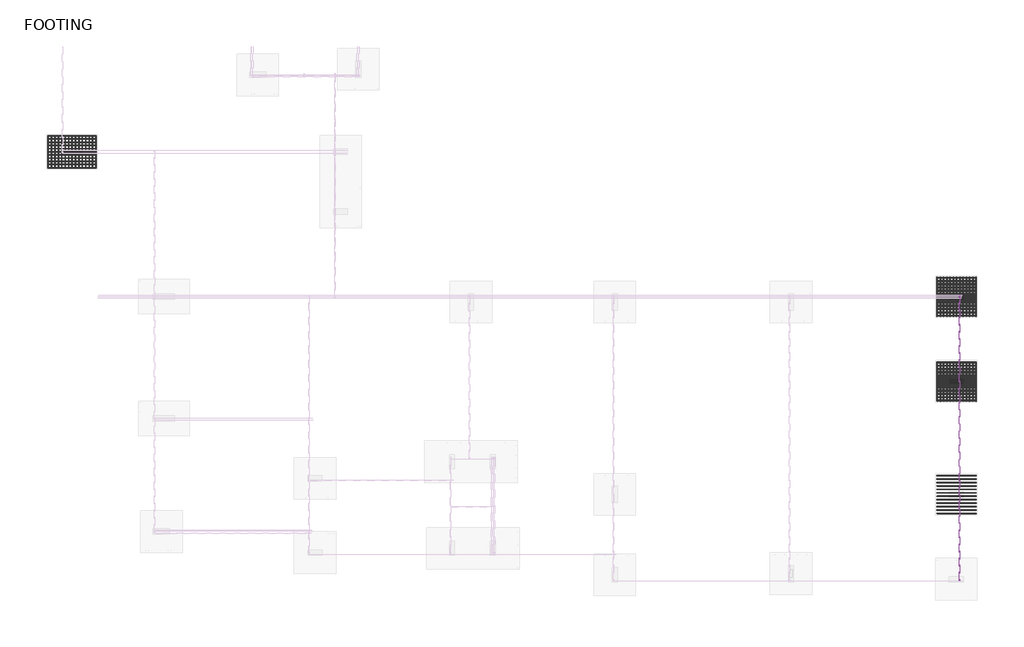
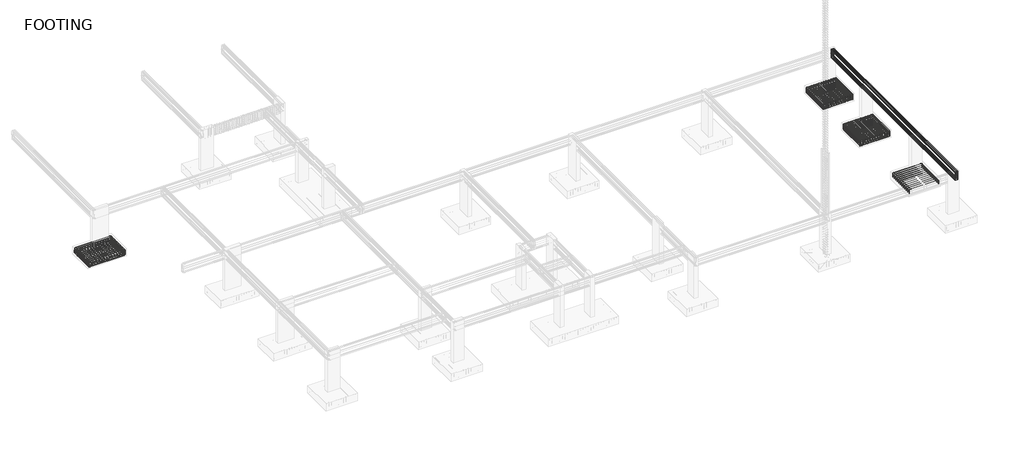
# One storey, part 9 of 12: 15 reinforcing bars.
"""IFC4 building model written with IfcOpenShell, lengths in millimetres."""

from ifc_helpers import new_model, si_unit, point, frame, origin, place, context, project, spatial, polyline, circle_curve, trimmed, segment, composite_curve, source, transform, mapped, element, save
from ifc_brep_helpers import swept_disk

model = new_model("IFC4")

# Units and contexts
model_context = context("Model", 3, world=origin())
ifc_project = project(units=[si_unit("LENGTHUNIT", "METRE", prefix="MILLI")], contexts=[model_context])

# Site, building, storey
site = spatial("IfcSite", under=ifc_project)
building = spatial("IfcBuilding", under=site)
storey = spatial("IfcBuildingStorey", under=building, Name="FOOTING", Elevation=-5638.8)

# Reinforcing bars
placement = place(None, origin())
reinforcing_bar_shape = source(origin(), model_context, "Body", "SolidModel", [
    swept_disk(composite_curve([segment(polyline([(18367.9998335, -9883.6399866, -5950.85), (18367.9998335, -9883.6399866, -5764.25)]), True, "CONTINUOUS"), segment(trimmed(circle_curve(frame((18423.4498335, -9883.6399866, -5764.25), z_axis=(0.0, 1.0, 0.0), x_axis=(-55.45000000000073, 0.0, 0.0)), 55.45), [point((18367.9998335, -9883.6399866, -5764.25))], [point((18423.4498335, -9883.6399866, -5708.8))], True, "CARTESIAN"), True, "CONTINUOUS"), segment(polyline([(18423.4498335, -9883.6399866, -5708.8), (19996.6498335, -9883.6399866, -5708.8)]), True, "CONTINUOUS"), segment(trimmed(circle_curve(frame((19996.6498335, -9883.6399866, -5764.25), z_axis=(0.0, 1.0, 0.0), x_axis=(0.0, 0.0, 55.44999999999982)), 55.45), [point((19996.6498335, -9883.6399866, -5708.8))], [point((20052.0998335, -9883.6399866, -5764.25))], True, "CARTESIAN"), True, "CONTINUOUS"), segment(polyline([(20052.0998335, -9883.6399866, -5764.25), (20052.0998335, -9883.6399866, -5950.85)]), True, "CONTINUOUS")], self_intersect=False), 7.95),
])
element("IfcReinforcingBar", 1, at=placement, inside=storey, context=model_context, shape_type="MappedRepresentation", body=[
    mapped(reinforcing_bar_shape, transform((0.0, 0.0, 0.0), x_axis=(1.0, 0.0, 0.0), y_axis=(0.0, 1.0, 0.0), z_axis=(0.0, 0.0, 1.0))),
    mapped(reinforcing_bar_shape, transform((0.0, -148.1882348, 0.0), x_axis=(1.0, 0.0, 0.0), y_axis=(0.0, 1.0, 0.0), z_axis=(0.0, 0.0, 1.0))),
    mapped(reinforcing_bar_shape, transform((0.0, -296.3764695, 0.0), x_axis=(1.0, 0.0, 0.0), y_axis=(0.0, 1.0, 0.0), z_axis=(0.0, 0.0, 1.0))),
    mapped(reinforcing_bar_shape, transform((0.0, -444.5647043, 0.0), x_axis=(1.0, 0.0, 0.0), y_axis=(0.0, 1.0, 0.0), z_axis=(0.0, 0.0, 1.0))),
    mapped(reinforcing_bar_shape, transform((0.0, -592.7529391, 0.0), x_axis=(1.0, 0.0, 0.0), y_axis=(0.0, 1.0, 0.0), z_axis=(0.0, 0.0, 1.0))),
    mapped(reinforcing_bar_shape, transform((0.0, -740.9411738, 0.0), x_axis=(1.0, 0.0, 0.0), y_axis=(0.0, 1.0, 0.0), z_axis=(0.0, 0.0, 1.0))),
    mapped(reinforcing_bar_shape, transform((0.0, -889.1294086, 0.0), x_axis=(1.0, 0.0, 0.0), y_axis=(0.0, 1.0, 0.0), z_axis=(0.0, 0.0, 1.0))),
    mapped(reinforcing_bar_shape, transform((0.0, -1037.3176434, 0.0), x_axis=(1.0, 0.0, 0.0), y_axis=(0.0, 1.0, 0.0), z_axis=(0.0, 0.0, 1.0))),
    mapped(reinforcing_bar_shape, transform((0.0, -1185.5058782, 0.0), x_axis=(1.0, 0.0, 0.0), y_axis=(0.0, 1.0, 0.0), z_axis=(0.0, 0.0, 1.0))),
    mapped(reinforcing_bar_shape, transform((0.0, -1333.6941129, 0.0), x_axis=(1.0, 0.0, 0.0), y_axis=(0.0, 1.0, 0.0), z_axis=(0.0, 0.0, 1.0))),
    mapped(reinforcing_bar_shape, transform((0.0, -1481.8823477, 0.0), x_axis=(1.0, 0.0, 0.0), y_axis=(0.0, 1.0, 0.0), z_axis=(0.0, 0.0, 1.0))),
    mapped(reinforcing_bar_shape, transform((0.0, -1630.0705825, 0.0), x_axis=(1.0, 0.0, 0.0), y_axis=(0.0, 1.0, 0.0), z_axis=(0.0, 0.0, 1.0))),
])
reinforcing_bar_2_shape = source(origin(), model_context, "Body", "SolidModel", [
    swept_disk(composite_curve([segment(polyline([(20052.0998335, -6666.5541655, -5788.8), (20052.0998335, -6666.5541655, -5975.4)]), True, "CONTINUOUS"), segment(trimmed(circle_curve(frame((20052.0998335, -6611.1041655, -5975.4), z_axis=(1.0, 0.0, 0.0), x_axis=(0.0, -55.44999999999982, 0.0)), 55.45), [point((20052.0998335, -6666.5541655, -5975.4))], [point((20052.0998335, -6611.1041655, -6030.85))], True, "CARTESIAN"), True, "CONTINUOUS"), segment(polyline([(20052.0998335, -6611.1041655, -6030.85), (20052.0998335, -5037.9041655, -6030.85)]), True, "CONTINUOUS"), segment(trimmed(circle_curve(frame((20052.0998335, -5037.9041655, -5975.4), z_axis=(1.0, 0.0, 0.0), x_axis=(0.0, 0.0, -55.45000000000073)), 55.45), [point((20052.0998335, -5037.9041655, -6030.85))], [point((20052.0998335, -4982.4541655, -5975.4))], True, "CARTESIAN"), True, "CONTINUOUS"), segment(polyline([(20052.0998335, -4982.4541655, -5975.4), (20052.0998335, -4982.4541655, -5788.8)]), True, "CONTINUOUS")], self_intersect=False), 7.95),
])
element("IfcReinforcingBar", 2, at=placement, inside=storey, context=model_context, shape_type="MappedRepresentation", body=[
    mapped(reinforcing_bar_2_shape, transform((0.0, 0.0, 0.0), x_axis=(1.0, 0.0, 0.0), y_axis=(0.0, 1.0, 0.0), z_axis=(0.0, 0.0, 1.0))),
    mapped(reinforcing_bar_2_shape, transform((-140.3416667, 0.0, 0.0), x_axis=(1.0, 0.0, 0.0), y_axis=(0.0, 1.0, 0.0), z_axis=(0.0, 0.0, 1.0))),
    mapped(reinforcing_bar_2_shape, transform((-280.6833333, 0.0, 0.0), x_axis=(1.0, 0.0, 0.0), y_axis=(0.0, 1.0, 0.0), z_axis=(0.0, 0.0, 1.0))),
    mapped(reinforcing_bar_2_shape, transform((-421.025, 0.0, 0.0), x_axis=(1.0, 0.0, 0.0), y_axis=(0.0, 1.0, 0.0), z_axis=(0.0, 0.0, 1.0))),
    mapped(reinforcing_bar_2_shape, transform((-561.3666667, 0.0, 0.0), x_axis=(1.0, 0.0, 0.0), y_axis=(0.0, 1.0, 0.0), z_axis=(0.0, 0.0, 1.0))),
    mapped(reinforcing_bar_2_shape, transform((-701.7083333, 0.0, 0.0), x_axis=(1.0, 0.0, 0.0), y_axis=(0.0, 1.0, 0.0), z_axis=(0.0, 0.0, 1.0))),
    mapped(reinforcing_bar_2_shape, transform((-842.05, 0.0, 0.0), x_axis=(1.0, 0.0, 0.0), y_axis=(0.0, 1.0, 0.0), z_axis=(0.0, 0.0, 1.0))),
    mapped(reinforcing_bar_2_shape, transform((-982.3916667, 0.0, 0.0), x_axis=(1.0, 0.0, 0.0), y_axis=(0.0, 1.0, 0.0), z_axis=(0.0, 0.0, 1.0))),
    mapped(reinforcing_bar_2_shape, transform((-1122.7333333, 0.0, 0.0), x_axis=(1.0, 0.0, 0.0), y_axis=(0.0, 1.0, 0.0), z_axis=(0.0, 0.0, 1.0))),
    mapped(reinforcing_bar_2_shape, transform((-1263.075, 0.0, 0.0), x_axis=(1.0, 0.0, 0.0), y_axis=(0.0, 1.0, 0.0), z_axis=(0.0, 0.0, 1.0))),
    mapped(reinforcing_bar_2_shape, transform((-1403.4166667, 0.0, 0.0), x_axis=(1.0, 0.0, 0.0), y_axis=(0.0, 1.0, 0.0), z_axis=(0.0, 0.0, 1.0))),
    mapped(reinforcing_bar_2_shape, transform((-1543.7583333, 0.0, 0.0), x_axis=(1.0, 0.0, 0.0), y_axis=(0.0, 1.0, 0.0), z_axis=(0.0, 0.0, 1.0))),
    mapped(reinforcing_bar_2_shape, transform((-1684.1, 0.0, 0.0), x_axis=(1.0, 0.0, 0.0), y_axis=(0.0, 1.0, 0.0), z_axis=(0.0, 0.0, 1.0))),
])
reinforcing_bar_3_shape = source(origin(), model_context, "Body", "SolidModel", [
    swept_disk(composite_curve([segment(polyline([(20042.9597994, -4980.8541655, -5888.8), (20042.9597994, -4980.8541655, -5741.5)]), True, "CONTINUOUS"), segment(trimmed(circle_curve(frame((20042.9597994, -5027.2041655, -5741.5), z_axis=(1.0, 0.0, 0.0), x_axis=(0.0, 46.350000000000364, 0.0)), 46.35), [point((20042.9597994, -4980.8541655, -5741.5))], [point((20042.9597994, -5027.2041655, -5695.15))], True, "CARTESIAN"), True, "CONTINUOUS"), segment(polyline([(20042.9597994, -5027.2041655, -5695.15), (20042.9597994, -6621.8041655, -5695.15)]), True, "CONTINUOUS"), segment(trimmed(circle_curve(frame((20042.9597994, -6621.8041655, -5741.5), z_axis=(1.0, 0.0, 0.0), x_axis=(0.0, 0.0, 46.350000000000364)), 46.35), [point((20042.9597994, -6621.8041655, -5695.15))], [point((20042.9597994, -6668.1541655, -5741.5))], True, "CARTESIAN"), True, "CONTINUOUS"), segment(polyline([(20042.9597994, -6668.1541655, -5741.5), (20042.9597994, -6668.1541655, -5888.8)]), True, "CONTINUOUS")], self_intersect=False), 6.35),
])
element("IfcReinforcingBar", 3, at=placement, inside=storey, context=model_context, shape_type="MappedRepresentation", body=[
    mapped(reinforcing_bar_3_shape, transform((0.0, 0.0, 0.0), x_axis=(1.0, 0.0, 0.0), y_axis=(0.0, 1.0, 0.0), z_axis=(0.0, 0.0, 1.0))),
    mapped(reinforcing_bar_3_shape, transform((-138.4829293, 0.0, 0.0), x_axis=(1.0, 0.0, 0.0), y_axis=(0.0, 1.0, 0.0), z_axis=(0.0, 0.0, 1.0))),
    mapped(reinforcing_bar_3_shape, transform((-276.9658586, 0.0, 0.0), x_axis=(1.0, 0.0, 0.0), y_axis=(0.0, 1.0, 0.0), z_axis=(0.0, 0.0, 1.0))),
    mapped(reinforcing_bar_3_shape, transform((-415.4487879, 0.0, 0.0), x_axis=(1.0, 0.0, 0.0), y_axis=(0.0, 1.0, 0.0), z_axis=(0.0, 0.0, 1.0))),
    mapped(reinforcing_bar_3_shape, transform((-553.9317172, 0.0, 0.0), x_axis=(1.0, 0.0, 0.0), y_axis=(0.0, 1.0, 0.0), z_axis=(0.0, 0.0, 1.0))),
    mapped(reinforcing_bar_3_shape, transform((-692.4146465, 0.0, 0.0), x_axis=(1.0, 0.0, 0.0), y_axis=(0.0, 1.0, 0.0), z_axis=(0.0, 0.0, 1.0))),
    mapped(reinforcing_bar_3_shape, transform((-830.8975758, 0.0, 0.0), x_axis=(1.0, 0.0, 0.0), y_axis=(0.0, 1.0, 0.0), z_axis=(0.0, 0.0, 1.0))),
    mapped(reinforcing_bar_3_shape, transform((-969.3805051, 0.0, 0.0), x_axis=(1.0, 0.0, 0.0), y_axis=(0.0, 1.0, 0.0), z_axis=(0.0, 0.0, 1.0))),
    mapped(reinforcing_bar_3_shape, transform((-1107.8634344, 0.0, 0.0), x_axis=(1.0, 0.0, 0.0), y_axis=(0.0, 1.0, 0.0), z_axis=(0.0, 0.0, 1.0))),
    mapped(reinforcing_bar_3_shape, transform((-1246.3463637, 0.0, 0.0), x_axis=(1.0, 0.0, 0.0), y_axis=(0.0, 1.0, 0.0), z_axis=(0.0, 0.0, 1.0))),
    mapped(reinforcing_bar_3_shape, transform((-1384.8292929, 0.0, 0.0), x_axis=(1.0, 0.0, 0.0), y_axis=(0.0, 1.0, 0.0), z_axis=(0.0, 0.0, 1.0))),
    mapped(reinforcing_bar_3_shape, transform((-1523.3122222, 0.0, 0.0), x_axis=(1.0, 0.0, 0.0), y_axis=(0.0, 1.0, 0.0), z_axis=(0.0, 0.0, 1.0))),
    mapped(reinforcing_bar_3_shape, transform((-1661.7951515, 0.0, 0.0), x_axis=(1.0, 0.0, 0.0), y_axis=(0.0, 1.0, 0.0), z_axis=(0.0, 0.0, 1.0))),
])
reinforcing_bar_4_shape = source(origin(), model_context, "Body", "SolidModel", [
    swept_disk(composite_curve([segment(polyline([(18367.9998335, -6649.5041655, -5773.0), (18367.9998335, -6649.5041655, -5959.6)]), True, "CONTINUOUS"), segment(trimmed(circle_curve(frame((18423.4498335, -6649.5041655, -5959.6), z_axis=(0.0, -1.0, 0.0), x_axis=(-55.45000000000073, 0.0, 0.0)), 55.45), [point((18367.9998335, -6649.5041655, -5959.6))], [point((18423.4498335, -6649.5041655, -6015.05))], True, "CARTESIAN"), True, "CONTINUOUS"), segment(polyline([(18423.4498335, -6649.5041655, -6015.05), (19996.6498335, -6649.5041655, -6015.05)]), True, "CONTINUOUS"), segment(trimmed(circle_curve(frame((19996.6498335, -6649.5041655, -5959.6), z_axis=(0.0, -1.0, 0.0), x_axis=(0.0, 0.0, -55.44999999999982)), 55.45), [point((19996.6498335, -6649.5041655, -6015.05))], [point((20052.0998335, -6649.5041655, -5959.6))], True, "CARTESIAN"), True, "CONTINUOUS"), segment(polyline([(20052.0998335, -6649.5041655, -5959.6), (20052.0998335, -6649.5041655, -5773.0)]), True, "CONTINUOUS")], self_intersect=False), 7.95),
])
element("IfcReinforcingBar", 4, at=placement, inside=storey, context=model_context, shape_type="MappedRepresentation", body=[
    mapped(reinforcing_bar_4_shape, transform((0.0, 0.0, 0.0), x_axis=(1.0, 0.0, 0.0), y_axis=(0.0, 1.0, 0.0), z_axis=(0.0, 0.0, 1.0))),
    mapped(reinforcing_bar_4_shape, transform((0.0, 137.7402087, 0.0), x_axis=(1.0, 0.0, 0.0), y_axis=(0.0, 1.0, 0.0), z_axis=(0.0, 0.0, 1.0))),
    mapped(reinforcing_bar_4_shape, transform((0.0, 275.4804175, 0.0), x_axis=(1.0, 0.0, 0.0), y_axis=(0.0, 1.0, 0.0), z_axis=(0.0, 0.0, 1.0))),
    mapped(reinforcing_bar_4_shape, transform((0.0, 413.2206262, 0.0), x_axis=(1.0, 0.0, 0.0), y_axis=(0.0, 1.0, 0.0), z_axis=(0.0, 0.0, 1.0))),
    mapped(reinforcing_bar_4_shape, transform((0.0, 550.960835, 0.0), x_axis=(1.0, 0.0, 0.0), y_axis=(0.0, 1.0, 0.0), z_axis=(0.0, 0.0, 1.0))),
    mapped(reinforcing_bar_4_shape, transform((0.0, 688.7010437, 0.0), x_axis=(1.0, 0.0, 0.0), y_axis=(0.0, 1.0, 0.0), z_axis=(0.0, 0.0, 1.0))),
    mapped(reinforcing_bar_4_shape, transform((0.0, 826.4412525, 0.0), x_axis=(1.0, 0.0, 0.0), y_axis=(0.0, 1.0, 0.0), z_axis=(0.0, 0.0, 1.0))),
    mapped(reinforcing_bar_4_shape, transform((0.0, 964.1814612, 0.0), x_axis=(1.0, 0.0, 0.0), y_axis=(0.0, 1.0, 0.0), z_axis=(0.0, 0.0, 1.0))),
    mapped(reinforcing_bar_4_shape, transform((0.0, 1101.92167, 0.0), x_axis=(1.0, 0.0, 0.0), y_axis=(0.0, 1.0, 0.0), z_axis=(0.0, 0.0, 1.0))),
    mapped(reinforcing_bar_4_shape, transform((0.0, 1239.6618787, 0.0), x_axis=(1.0, 0.0, 0.0), y_axis=(0.0, 1.0, 0.0), z_axis=(0.0, 0.0, 1.0))),
    mapped(reinforcing_bar_4_shape, transform((0.0, 1377.4020875, 0.0), x_axis=(1.0, 0.0, 0.0), y_axis=(0.0, 1.0, 0.0), z_axis=(0.0, 0.0, 1.0))),
    mapped(reinforcing_bar_4_shape, transform((0.0, 1515.1422962, 0.0), x_axis=(1.0, 0.0, 0.0), y_axis=(0.0, 1.0, 0.0), z_axis=(0.0, 0.0, 1.0))),
    mapped(reinforcing_bar_4_shape, transform((0.0, 1652.882505, 0.0), x_axis=(1.0, 0.0, 0.0), y_axis=(0.0, 1.0, 0.0), z_axis=(0.0, 0.0, 1.0))),
])
reinforcing_bar_5_shape = source(origin(), model_context, "Body", "SolidModel", [
    swept_disk(composite_curve([segment(polyline([(18367.9998335, -5006.8399866, -5950.85), (18367.9998335, -5006.8399866, -5764.25)]), True, "CONTINUOUS"), segment(trimmed(circle_curve(frame((18423.4498335, -5006.8399866, -5764.25), z_axis=(0.0, 1.0, 0.0), x_axis=(-55.45000000000073, 0.0, 0.0)), 55.45), [point((18367.9998335, -5006.8399866, -5764.25))], [point((18423.4498335, -5006.8399866, -5708.8))], True, "CARTESIAN"), True, "CONTINUOUS"), segment(polyline([(18423.4498335, -5006.8399866, -5708.8), (19996.6498335, -5006.8399866, -5708.8)]), True, "CONTINUOUS"), segment(trimmed(circle_curve(frame((19996.6498335, -5006.8399866, -5764.25), z_axis=(0.0, 1.0, 0.0), x_axis=(0.0, 0.0, 55.44999999999982)), 55.45), [point((19996.6498335, -5006.8399866, -5708.8))], [point((20052.0998335, -5006.8399866, -5764.25))], True, "CARTESIAN"), True, "CONTINUOUS"), segment(polyline([(20052.0998335, -5006.8399866, -5764.25), (20052.0998335, -5006.8399866, -5950.85)]), True, "CONTINUOUS")], self_intersect=False), 7.95),
])
element("IfcReinforcingBar", 5, at=placement, inside=storey, context=model_context, shape_type="MappedRepresentation", body=[
    mapped(reinforcing_bar_5_shape, transform((0.0, 0.0, 0.0), x_axis=(1.0, 0.0, 0.0), y_axis=(0.0, 1.0, 0.0), z_axis=(0.0, 0.0, 1.0))),
    mapped(reinforcing_bar_5_shape, transform((0.0, -148.1882348, 0.0), x_axis=(1.0, 0.0, 0.0), y_axis=(0.0, 1.0, 0.0), z_axis=(0.0, 0.0, 1.0))),
    mapped(reinforcing_bar_5_shape, transform((0.0, -296.3764695, 0.0), x_axis=(1.0, 0.0, 0.0), y_axis=(0.0, 1.0, 0.0), z_axis=(0.0, 0.0, 1.0))),
    mapped(reinforcing_bar_5_shape, transform((0.0, -444.5647043, 0.0), x_axis=(1.0, 0.0, 0.0), y_axis=(0.0, 1.0, 0.0), z_axis=(0.0, 0.0, 1.0))),
    mapped(reinforcing_bar_5_shape, transform((0.0, -592.7529391, 0.0), x_axis=(1.0, 0.0, 0.0), y_axis=(0.0, 1.0, 0.0), z_axis=(0.0, 0.0, 1.0))),
    mapped(reinforcing_bar_5_shape, transform((0.0, -740.9411738, 0.0), x_axis=(1.0, 0.0, 0.0), y_axis=(0.0, 1.0, 0.0), z_axis=(0.0, 0.0, 1.0))),
    mapped(reinforcing_bar_5_shape, transform((0.0, -889.1294086, 0.0), x_axis=(1.0, 0.0, 0.0), y_axis=(0.0, 1.0, 0.0), z_axis=(0.0, 0.0, 1.0))),
    mapped(reinforcing_bar_5_shape, transform((0.0, -1037.3176434, 0.0), x_axis=(1.0, 0.0, 0.0), y_axis=(0.0, 1.0, 0.0), z_axis=(0.0, 0.0, 1.0))),
    mapped(reinforcing_bar_5_shape, transform((0.0, -1185.5058782, 0.0), x_axis=(1.0, 0.0, 0.0), y_axis=(0.0, 1.0, 0.0), z_axis=(0.0, 0.0, 1.0))),
    mapped(reinforcing_bar_5_shape, transform((0.0, -1333.6941129, 0.0), x_axis=(1.0, 0.0, 0.0), y_axis=(0.0, 1.0, 0.0), z_axis=(0.0, 0.0, 1.0))),
    mapped(reinforcing_bar_5_shape, transform((0.0, -1481.8823477, 0.0), x_axis=(1.0, 0.0, 0.0), y_axis=(0.0, 1.0, 0.0), z_axis=(0.0, 0.0, 1.0))),
    mapped(reinforcing_bar_5_shape, transform((0.0, -1630.0705825, 0.0), x_axis=(1.0, 0.0, 0.0), y_axis=(0.0, 1.0, 0.0), z_axis=(0.0, 0.0, 1.0))),
])
reinforcing_bar_6_shape = source(origin(), model_context, "Body", "SolidModel", [
    swept_disk(composite_curve([segment(polyline([(20052.0998335, -3008.9541655, -5788.8), (20052.0998335, -3008.9541655, -5975.4)]), True, "CONTINUOUS"), segment(trimmed(circle_curve(frame((20052.0998335, -2953.5041655, -5975.4), z_axis=(1.0, 0.0, 0.0), x_axis=(0.0, -55.44999999999982, 0.0)), 55.45), [point((20052.0998335, -3008.9541655, -5975.4))], [point((20052.0998335, -2953.5041655, -6030.85))], True, "CARTESIAN"), True, "CONTINUOUS"), segment(polyline([(20052.0998335, -2953.5041655, -6030.85), (20052.0998335, -1380.3041655, -6030.85)]), True, "CONTINUOUS"), segment(trimmed(circle_curve(frame((20052.0998335, -1380.3041655, -5975.4), z_axis=(1.0, 0.0, 0.0), x_axis=(0.0, 0.0, -55.45000000000073)), 55.45), [point((20052.0998335, -1380.3041655, -6030.85))], [point((20052.0998335, -1324.8541655, -5975.4))], True, "CARTESIAN"), True, "CONTINUOUS"), segment(polyline([(20052.0998335, -1324.8541655, -5975.4), (20052.0998335, -1324.8541655, -5788.8)]), True, "CONTINUOUS")], self_intersect=False), 7.95),
])
element("IfcReinforcingBar", 6, at=placement, inside=storey, context=model_context, shape_type="MappedRepresentation", body=[
    mapped(reinforcing_bar_6_shape, transform((0.0, 0.0, 0.0), x_axis=(1.0, 0.0, 0.0), y_axis=(0.0, 1.0, 0.0), z_axis=(0.0, 0.0, 1.0))),
    mapped(reinforcing_bar_6_shape, transform((-140.3416667, 0.0, 0.0), x_axis=(1.0, 0.0, 0.0), y_axis=(0.0, 1.0, 0.0), z_axis=(0.0, 0.0, 1.0))),
    mapped(reinforcing_bar_6_shape, transform((-280.6833333, 0.0, 0.0), x_axis=(1.0, 0.0, 0.0), y_axis=(0.0, 1.0, 0.0), z_axis=(0.0, 0.0, 1.0))),
    mapped(reinforcing_bar_6_shape, transform((-421.025, 0.0, 0.0), x_axis=(1.0, 0.0, 0.0), y_axis=(0.0, 1.0, 0.0), z_axis=(0.0, 0.0, 1.0))),
    mapped(reinforcing_bar_6_shape, transform((-561.3666667, 0.0, 0.0), x_axis=(1.0, 0.0, 0.0), y_axis=(0.0, 1.0, 0.0), z_axis=(0.0, 0.0, 1.0))),
    mapped(reinforcing_bar_6_shape, transform((-701.7083333, 0.0, 0.0), x_axis=(1.0, 0.0, 0.0), y_axis=(0.0, 1.0, 0.0), z_axis=(0.0, 0.0, 1.0))),
    mapped(reinforcing_bar_6_shape, transform((-842.05, 0.0, 0.0), x_axis=(1.0, 0.0, 0.0), y_axis=(0.0, 1.0, 0.0), z_axis=(0.0, 0.0, 1.0))),
    mapped(reinforcing_bar_6_shape, transform((-982.3916667, 0.0, 0.0), x_axis=(1.0, 0.0, 0.0), y_axis=(0.0, 1.0, 0.0), z_axis=(0.0, 0.0, 1.0))),
    mapped(reinforcing_bar_6_shape, transform((-1122.7333333, 0.0, 0.0), x_axis=(1.0, 0.0, 0.0), y_axis=(0.0, 1.0, 0.0), z_axis=(0.0, 0.0, 1.0))),
    mapped(reinforcing_bar_6_shape, transform((-1263.075, 0.0, 0.0), x_axis=(1.0, 0.0, 0.0), y_axis=(0.0, 1.0, 0.0), z_axis=(0.0, 0.0, 1.0))),
    mapped(reinforcing_bar_6_shape, transform((-1403.4166667, 0.0, 0.0), x_axis=(1.0, 0.0, 0.0), y_axis=(0.0, 1.0, 0.0), z_axis=(0.0, 0.0, 1.0))),
    mapped(reinforcing_bar_6_shape, transform((-1543.7583333, 0.0, 0.0), x_axis=(1.0, 0.0, 0.0), y_axis=(0.0, 1.0, 0.0), z_axis=(0.0, 0.0, 1.0))),
    mapped(reinforcing_bar_6_shape, transform((-1684.1, 0.0, 0.0), x_axis=(1.0, 0.0, 0.0), y_axis=(0.0, 1.0, 0.0), z_axis=(0.0, 0.0, 1.0))),
])
reinforcing_bar_7_shape = source(origin(), model_context, "Body", "SolidModel", [
    swept_disk(composite_curve([segment(polyline([(20042.9597994, -1323.2541655, -5888.8), (20042.9597994, -1323.2541655, -5741.5)]), True, "CONTINUOUS"), segment(trimmed(circle_curve(frame((20042.9597994, -1369.6041655, -5741.5), z_axis=(1.0, 0.0, 0.0), x_axis=(0.0, 46.34999999999991, 0.0)), 46.35), [point((20042.9597994, -1323.2541655, -5741.5))], [point((20042.9597994, -1369.6041655, -5695.15))], True, "CARTESIAN"), True, "CONTINUOUS"), segment(polyline([(20042.9597994, -1369.6041655, -5695.15), (20042.9597994, -2964.2041655, -5695.15)]), True, "CONTINUOUS"), segment(trimmed(circle_curve(frame((20042.9597994, -2964.2041655, -5741.5), z_axis=(1.0, 0.0, 0.0), x_axis=(0.0, 0.0, 46.350000000000364)), 46.35), [point((20042.9597994, -2964.2041655, -5695.15))], [point((20042.9597994, -3010.5541655, -5741.5))], True, "CARTESIAN"), True, "CONTINUOUS"), segment(polyline([(20042.9597994, -3010.5541655, -5741.5), (20042.9597994, -3010.5541655, -5888.8)]), True, "CONTINUOUS")], self_intersect=False), 6.35),
])
element("IfcReinforcingBar", 7, at=placement, inside=storey, context=model_context, shape_type="MappedRepresentation", body=[
    mapped(reinforcing_bar_7_shape, transform((0.0, 0.0, 0.0), x_axis=(1.0, 0.0, 0.0), y_axis=(0.0, 1.0, 0.0), z_axis=(0.0, 0.0, 1.0))),
    mapped(reinforcing_bar_7_shape, transform((-138.4829293, 0.0, 0.0), x_axis=(1.0, 0.0, 0.0), y_axis=(0.0, 1.0, 0.0), z_axis=(0.0, 0.0, 1.0))),
    mapped(reinforcing_bar_7_shape, transform((-276.9658586, 0.0, 0.0), x_axis=(1.0, 0.0, 0.0), y_axis=(0.0, 1.0, 0.0), z_axis=(0.0, 0.0, 1.0))),
    mapped(reinforcing_bar_7_shape, transform((-415.4487879, 0.0, 0.0), x_axis=(1.0, 0.0, 0.0), y_axis=(0.0, 1.0, 0.0), z_axis=(0.0, 0.0, 1.0))),
    mapped(reinforcing_bar_7_shape, transform((-553.9317172, 0.0, 0.0), x_axis=(1.0, 0.0, 0.0), y_axis=(0.0, 1.0, 0.0), z_axis=(0.0, 0.0, 1.0))),
    mapped(reinforcing_bar_7_shape, transform((-692.4146465, 0.0, 0.0), x_axis=(1.0, 0.0, 0.0), y_axis=(0.0, 1.0, 0.0), z_axis=(0.0, 0.0, 1.0))),
    mapped(reinforcing_bar_7_shape, transform((-830.8975758, 0.0, 0.0), x_axis=(1.0, 0.0, 0.0), y_axis=(0.0, 1.0, 0.0), z_axis=(0.0, 0.0, 1.0))),
    mapped(reinforcing_bar_7_shape, transform((-969.3805051, 0.0, 0.0), x_axis=(1.0, 0.0, 0.0), y_axis=(0.0, 1.0, 0.0), z_axis=(0.0, 0.0, 1.0))),
    mapped(reinforcing_bar_7_shape, transform((-1107.8634344, 0.0, 0.0), x_axis=(1.0, 0.0, 0.0), y_axis=(0.0, 1.0, 0.0), z_axis=(0.0, 0.0, 1.0))),
    mapped(reinforcing_bar_7_shape, transform((-1246.3463637, 0.0, 0.0), x_axis=(1.0, 0.0, 0.0), y_axis=(0.0, 1.0, 0.0), z_axis=(0.0, 0.0, 1.0))),
    mapped(reinforcing_bar_7_shape, transform((-1384.8292929, 0.0, 0.0), x_axis=(1.0, 0.0, 0.0), y_axis=(0.0, 1.0, 0.0), z_axis=(0.0, 0.0, 1.0))),
    mapped(reinforcing_bar_7_shape, transform((-1523.3122222, 0.0, 0.0), x_axis=(1.0, 0.0, 0.0), y_axis=(0.0, 1.0, 0.0), z_axis=(0.0, 0.0, 1.0))),
    mapped(reinforcing_bar_7_shape, transform((-1661.7951515, 0.0, 0.0), x_axis=(1.0, 0.0, 0.0), y_axis=(0.0, 1.0, 0.0), z_axis=(0.0, 0.0, 1.0))),
])
reinforcing_bar_8_shape = source(origin(), model_context, "Body", "SolidModel", [
    swept_disk(composite_curve([segment(polyline([(18367.9998335, -2991.9041655, -5773.0), (18367.9998335, -2991.9041655, -5959.6)]), True, "CONTINUOUS"), segment(trimmed(circle_curve(frame((18423.4498335, -2991.9041655, -5959.6), z_axis=(0.0, -1.0, 0.0), x_axis=(-55.45000000000073, 0.0, 0.0)), 55.45), [point((18367.9998335, -2991.9041655, -5959.6))], [point((18423.4498335, -2991.9041655, -6015.05))], True, "CARTESIAN"), True, "CONTINUOUS"), segment(polyline([(18423.4498335, -2991.9041655, -6015.05), (19996.6498335, -2991.9041655, -6015.05)]), True, "CONTINUOUS"), segment(trimmed(circle_curve(frame((19996.6498335, -2991.9041655, -5959.6), z_axis=(0.0, -1.0, 0.0), x_axis=(0.0, 0.0, -55.44999999999982)), 55.45), [point((19996.6498335, -2991.9041655, -6015.05))], [point((20052.0998335, -2991.9041655, -5959.6))], True, "CARTESIAN"), True, "CONTINUOUS"), segment(polyline([(20052.0998335, -2991.9041655, -5959.6), (20052.0998335, -2991.9041655, -5773.0)]), True, "CONTINUOUS")], self_intersect=False), 7.95),
])
element("IfcReinforcingBar", 8, at=placement, inside=storey, context=model_context, shape_type="MappedRepresentation", body=[
    mapped(reinforcing_bar_8_shape, transform((0.0, 0.0, 0.0), x_axis=(1.0, 0.0, 0.0), y_axis=(0.0, 1.0, 0.0), z_axis=(0.0, 0.0, 1.0))),
    mapped(reinforcing_bar_8_shape, transform((0.0, 137.7402087, 0.0), x_axis=(1.0, 0.0, 0.0), y_axis=(0.0, 1.0, 0.0), z_axis=(0.0, 0.0, 1.0))),
    mapped(reinforcing_bar_8_shape, transform((0.0, 275.4804175, 0.0), x_axis=(1.0, 0.0, 0.0), y_axis=(0.0, 1.0, 0.0), z_axis=(0.0, 0.0, 1.0))),
    mapped(reinforcing_bar_8_shape, transform((0.0, 413.2206262, 0.0), x_axis=(1.0, 0.0, 0.0), y_axis=(0.0, 1.0, 0.0), z_axis=(0.0, 0.0, 1.0))),
    mapped(reinforcing_bar_8_shape, transform((0.0, 550.960835, 0.0), x_axis=(1.0, 0.0, 0.0), y_axis=(0.0, 1.0, 0.0), z_axis=(0.0, 0.0, 1.0))),
    mapped(reinforcing_bar_8_shape, transform((0.0, 688.7010437, 0.0), x_axis=(1.0, 0.0, 0.0), y_axis=(0.0, 1.0, 0.0), z_axis=(0.0, 0.0, 1.0))),
    mapped(reinforcing_bar_8_shape, transform((0.0, 826.4412525, 0.0), x_axis=(1.0, 0.0, 0.0), y_axis=(0.0, 1.0, 0.0), z_axis=(0.0, 0.0, 1.0))),
    mapped(reinforcing_bar_8_shape, transform((0.0, 964.1814612, 0.0), x_axis=(1.0, 0.0, 0.0), y_axis=(0.0, 1.0, 0.0), z_axis=(0.0, 0.0, 1.0))),
    mapped(reinforcing_bar_8_shape, transform((0.0, 1101.92167, 0.0), x_axis=(1.0, 0.0, 0.0), y_axis=(0.0, 1.0, 0.0), z_axis=(0.0, 0.0, 1.0))),
    mapped(reinforcing_bar_8_shape, transform((0.0, 1239.6618787, 0.0), x_axis=(1.0, 0.0, 0.0), y_axis=(0.0, 1.0, 0.0), z_axis=(0.0, 0.0, 1.0))),
    mapped(reinforcing_bar_8_shape, transform((0.0, 1377.4020875, 0.0), x_axis=(1.0, 0.0, 0.0), y_axis=(0.0, 1.0, 0.0), z_axis=(0.0, 0.0, 1.0))),
    mapped(reinforcing_bar_8_shape, transform((0.0, 1515.1422962, 0.0), x_axis=(1.0, 0.0, 0.0), y_axis=(0.0, 1.0, 0.0), z_axis=(0.0, 0.0, 1.0))),
    mapped(reinforcing_bar_8_shape, transform((0.0, 1652.882505, 0.0), x_axis=(1.0, 0.0, 0.0), y_axis=(0.0, 1.0, 0.0), z_axis=(0.0, 0.0, 1.0))),
])
reinforcing_bar_9_shape = source(origin(), model_context, "Body", "SolidModel", [
    swept_disk(composite_curve([segment(polyline([(18367.9998335, -1349.2399866, -5950.85), (18367.9998335, -1349.2399866, -5764.25)]), True, "CONTINUOUS"), segment(trimmed(circle_curve(frame((18423.4498335, -1349.2399866, -5764.25), z_axis=(0.0, 1.0, 0.0), x_axis=(-55.45000000000073, 0.0, 0.0)), 55.45), [point((18367.9998335, -1349.2399866, -5764.25))], [point((18423.4498335, -1349.2399866, -5708.8))], True, "CARTESIAN"), True, "CONTINUOUS"), segment(polyline([(18423.4498335, -1349.2399866, -5708.8), (19996.6498335, -1349.2399866, -5708.8)]), True, "CONTINUOUS"), segment(trimmed(circle_curve(frame((19996.6498335, -1349.2399866, -5764.25), z_axis=(0.0, 1.0, 0.0), x_axis=(0.0, 0.0, 55.44999999999982)), 55.45), [point((19996.6498335, -1349.2399866, -5708.8))], [point((20052.0998335, -1349.2399866, -5764.25))], True, "CARTESIAN"), True, "CONTINUOUS"), segment(polyline([(20052.0998335, -1349.2399866, -5764.25), (20052.0998335, -1349.2399866, -5950.85)]), True, "CONTINUOUS")], self_intersect=False), 7.95),
])
element("IfcReinforcingBar", 9, at=placement, inside=storey, context=model_context, shape_type="MappedRepresentation", body=[
    mapped(reinforcing_bar_9_shape, transform((0.0, 0.0, 0.0), x_axis=(1.0, 0.0, 0.0), y_axis=(0.0, 1.0, 0.0), z_axis=(0.0, 0.0, 1.0))),
    mapped(reinforcing_bar_9_shape, transform((0.0, -148.1882348, 0.0), x_axis=(1.0, 0.0, 0.0), y_axis=(0.0, 1.0, 0.0), z_axis=(0.0, 0.0, 1.0))),
    mapped(reinforcing_bar_9_shape, transform((0.0, -296.3764695, 0.0), x_axis=(1.0, 0.0, 0.0), y_axis=(0.0, 1.0, 0.0), z_axis=(0.0, 0.0, 1.0))),
    mapped(reinforcing_bar_9_shape, transform((0.0, -444.5647043, 0.0), x_axis=(1.0, 0.0, 0.0), y_axis=(0.0, 1.0, 0.0), z_axis=(0.0, 0.0, 1.0))),
    mapped(reinforcing_bar_9_shape, transform((0.0, -592.7529391, 0.0), x_axis=(1.0, 0.0, 0.0), y_axis=(0.0, 1.0, 0.0), z_axis=(0.0, 0.0, 1.0))),
    mapped(reinforcing_bar_9_shape, transform((0.0, -740.9411738, 0.0), x_axis=(1.0, 0.0, 0.0), y_axis=(0.0, 1.0, 0.0), z_axis=(0.0, 0.0, 1.0))),
    mapped(reinforcing_bar_9_shape, transform((0.0, -889.1294086, 0.0), x_axis=(1.0, 0.0, 0.0), y_axis=(0.0, 1.0, 0.0), z_axis=(0.0, 0.0, 1.0))),
    mapped(reinforcing_bar_9_shape, transform((0.0, -1037.3176434, 0.0), x_axis=(1.0, 0.0, 0.0), y_axis=(0.0, 1.0, 0.0), z_axis=(0.0, 0.0, 1.0))),
    mapped(reinforcing_bar_9_shape, transform((0.0, -1185.5058782, 0.0), x_axis=(1.0, 0.0, 0.0), y_axis=(0.0, 1.0, 0.0), z_axis=(0.0, 0.0, 1.0))),
    mapped(reinforcing_bar_9_shape, transform((0.0, -1333.6941129, 0.0), x_axis=(1.0, 0.0, 0.0), y_axis=(0.0, 1.0, 0.0), z_axis=(0.0, 0.0, 1.0))),
    mapped(reinforcing_bar_9_shape, transform((0.0, -1481.8823477, 0.0), x_axis=(1.0, 0.0, 0.0), y_axis=(0.0, 1.0, 0.0), z_axis=(0.0, 0.0, 1.0))),
    mapped(reinforcing_bar_9_shape, transform((0.0, -1630.0705825, 0.0), x_axis=(1.0, 0.0, 0.0), y_axis=(0.0, 1.0, 0.0), z_axis=(0.0, 0.0, 1.0))),
])
reinforcing_bar_10_shape = source(origin(), model_context, "Body", "SolidModel", [
    swept_disk(composite_curve([segment(polyline([(-19946.3001665, 3387.8458345, -5837.6659404), (-19946.3001665, 3387.8458345, -5984.9659404)]), True, "CONTINUOUS"), segment(trimmed(circle_curve(frame((-19899.9501665, 3387.8458345, -5984.9659404), z_axis=(0.0, -1.0, 0.0), x_axis=(-46.35000000000218, 0.0, 0.0)), 46.35), [point((-19946.3001665, 3387.8458345, -5984.9659404))], [point((-19899.9501665, 3387.8458345, -6031.3159404))], True, "CARTESIAN"), True, "CONTINUOUS"), segment(polyline([(-19899.9501665, 3387.8458345, -6031.3159404), (-17905.3501665, 3387.8458345, -6031.3159404)]), True, "CONTINUOUS"), segment(trimmed(circle_curve(frame((-17905.3501665, 3387.8458345, -5984.9659404), z_axis=(0.0, -1.0, 0.0), x_axis=(0.0, 0.0, -46.349999999999454)), 46.35), [point((-17905.3501665, 3387.8458345, -6031.3159404))], [point((-17859.0001665, 3387.8458345, -5984.9659404))], True, "CARTESIAN"), True, "CONTINUOUS"), segment(polyline([(-17859.0001665, 3387.8458345, -5984.9659404), (-17859.0001665, 3387.8458345, -5837.6659404)]), True, "CONTINUOUS")], self_intersect=False), 6.35),
])
element("IfcReinforcingBar", 10, at=placement, inside=storey, context=model_context, shape_type="MappedRepresentation", body=[
    mapped(reinforcing_bar_10_shape, transform((0.0, 0.0, 0.0), x_axis=(1.0, 0.0, 0.0), y_axis=(0.0, 1.0, 0.0), z_axis=(0.0, 0.0, 1.0))),
    mapped(reinforcing_bar_10_shape, transform((0.0, 138.73, 0.0), x_axis=(1.0, 0.0, 0.0), y_axis=(0.0, 1.0, 0.0), z_axis=(0.0, 0.0, 1.0))),
    mapped(reinforcing_bar_10_shape, transform((0.0, 277.46, 0.0), x_axis=(1.0, 0.0, 0.0), y_axis=(0.0, 1.0, 0.0), z_axis=(0.0, 0.0, 1.0))),
    mapped(reinforcing_bar_10_shape, transform((0.0, 416.19, 0.0), x_axis=(1.0, 0.0, 0.0), y_axis=(0.0, 1.0, 0.0), z_axis=(0.0, 0.0, 1.0))),
    mapped(reinforcing_bar_10_shape, transform((0.0, 554.92, 0.0), x_axis=(1.0, 0.0, 0.0), y_axis=(0.0, 1.0, 0.0), z_axis=(0.0, 0.0, 1.0))),
    mapped(reinforcing_bar_10_shape, transform((0.0, 693.65, 0.0), x_axis=(1.0, 0.0, 0.0), y_axis=(0.0, 1.0, 0.0), z_axis=(0.0, 0.0, 1.0))),
    mapped(reinforcing_bar_10_shape, transform((0.0, 832.38, 0.0), x_axis=(1.0, 0.0, 0.0), y_axis=(0.0, 1.0, 0.0), z_axis=(0.0, 0.0, 1.0))),
    mapped(reinforcing_bar_10_shape, transform((0.0, 971.11, 0.0), x_axis=(1.0, 0.0, 0.0), y_axis=(0.0, 1.0, 0.0), z_axis=(0.0, 0.0, 1.0))),
    mapped(reinforcing_bar_10_shape, transform((0.0, 1109.84, 0.0), x_axis=(1.0, 0.0, 0.0), y_axis=(0.0, 1.0, 0.0), z_axis=(0.0, 0.0, 1.0))),
    mapped(reinforcing_bar_10_shape, transform((0.0, 1248.57, 0.0), x_axis=(1.0, 0.0, 0.0), y_axis=(0.0, 1.0, 0.0), z_axis=(0.0, 0.0, 1.0))),
    mapped(reinforcing_bar_10_shape, transform((0.0, 1387.3, 0.0), x_axis=(1.0, 0.0, 0.0), y_axis=(0.0, 1.0, 0.0), z_axis=(0.0, 0.0, 1.0))),
])
reinforcing_bar_11_shape = source(origin(), model_context, "Body", "SolidModel", [
    swept_disk(composite_curve([segment(polyline([(-17859.0001665, 3400.6454807, -5888.8), (-17859.0001665, 3400.6454807, -5741.5)]), True, "CONTINUOUS"), segment(trimmed(circle_curve(frame((-17905.3501665, 3400.6454807, -5741.5), z_axis=(0.0, -1.0, 0.0), x_axis=(46.349999999998545, 0.0, 0.0)), 46.35), [point((-17859.0001665, 3400.6454807, -5741.5))], [point((-17905.3501665, 3400.6454807, -5695.15))], True, "CARTESIAN"), True, "CONTINUOUS"), segment(polyline([(-17905.3501665, 3400.6454807, -5695.15), (-19899.9501665, 3400.6454807, -5695.15)]), True, "CONTINUOUS"), segment(trimmed(circle_curve(frame((-19899.9501665, 3400.6454807, -5741.5), z_axis=(0.0, -1.0, 0.0), x_axis=(0.0, 0.0, 46.350000000000364)), 46.35), [point((-19899.9501665, 3400.6454807, -5695.15))], [point((-19946.3001665, 3400.6454807, -5741.5))], True, "CARTESIAN"), True, "CONTINUOUS"), segment(polyline([(-19946.3001665, 3400.6454807, -5741.5), (-19946.3001665, 3400.6454807, -5888.8)]), True, "CONTINUOUS")], self_intersect=False), 6.35),
])
element("IfcReinforcingBar", 11, at=placement, inside=storey, context=model_context, shape_type="MappedRepresentation", body=[
    mapped(reinforcing_bar_11_shape, transform((0.0, 0.0, 0.0), x_axis=(1.0, 0.0, 0.0), y_axis=(0.0, 1.0, 0.0), z_axis=(0.0, 0.0, 1.0))),
    mapped(reinforcing_bar_11_shape, transform((0.0, 136.1586067, 0.0), x_axis=(1.0, 0.0, 0.0), y_axis=(0.0, 1.0, 0.0), z_axis=(0.0, 0.0, 1.0))),
    mapped(reinforcing_bar_11_shape, transform((0.0, 272.3172133, 0.0), x_axis=(1.0, 0.0, 0.0), y_axis=(0.0, 1.0, 0.0), z_axis=(0.0, 0.0, 1.0))),
    mapped(reinforcing_bar_11_shape, transform((0.0, 408.47582, 0.0), x_axis=(1.0, 0.0, 0.0), y_axis=(0.0, 1.0, 0.0), z_axis=(0.0, 0.0, 1.0))),
    mapped(reinforcing_bar_11_shape, transform((0.0, 544.6344267, 0.0), x_axis=(1.0, 0.0, 0.0), y_axis=(0.0, 1.0, 0.0), z_axis=(0.0, 0.0, 1.0))),
    mapped(reinforcing_bar_11_shape, transform((0.0, 680.7930333, 0.0), x_axis=(1.0, 0.0, 0.0), y_axis=(0.0, 1.0, 0.0), z_axis=(0.0, 0.0, 1.0))),
    mapped(reinforcing_bar_11_shape, transform((0.0, 816.95164, 0.0), x_axis=(1.0, 0.0, 0.0), y_axis=(0.0, 1.0, 0.0), z_axis=(0.0, 0.0, 1.0))),
    mapped(reinforcing_bar_11_shape, transform((0.0, 953.1102467, 0.0), x_axis=(1.0, 0.0, 0.0), y_axis=(0.0, 1.0, 0.0), z_axis=(0.0, 0.0, 1.0))),
    mapped(reinforcing_bar_11_shape, transform((0.0, 1089.2688533, 0.0), x_axis=(1.0, 0.0, 0.0), y_axis=(0.0, 1.0, 0.0), z_axis=(0.0, 0.0, 1.0))),
    mapped(reinforcing_bar_11_shape, transform((0.0, 1225.42746, 0.0), x_axis=(1.0, 0.0, 0.0), y_axis=(0.0, 1.0, 0.0), z_axis=(0.0, 0.0, 1.0))),
    mapped(reinforcing_bar_11_shape, transform((0.0, 1361.5860667, 0.0), x_axis=(1.0, 0.0, 0.0), y_axis=(0.0, 1.0, 0.0), z_axis=(0.0, 0.0, 1.0))),
])
reinforcing_bar_12_shape = source(origin(), model_context, "Body", "SolidModel", [
    swept_disk(composite_curve([segment(polyline([(-19934.3866414, 4775.1458345, -5821.490176), (-19934.3866414, 4775.1458345, -5968.790176)]), True, "CONTINUOUS"), segment(trimmed(circle_curve(frame((-19934.3866414, 4728.7958345, -5968.790176), z_axis=(-1.0, 0.0, 0.0), x_axis=(0.0, 46.350000000000364, 0.0)), 46.35), [point((-19934.3866414, 4775.1458345, -5968.790176))], [point((-19934.3866414, 4728.7958345, -6015.140176))], True, "CARTESIAN"), True, "CONTINUOUS"), segment(polyline([(-19934.3866414, 4728.7958345, -6015.140176), (-19934.3866414, 3434.1958345, -6015.140176)]), True, "CONTINUOUS"), segment(trimmed(circle_curve(frame((-19934.3866414, 3434.1958345, -5968.790176), z_axis=(-1.0, 0.0, 0.0), x_axis=(0.0, 0.0, -46.349999999999454)), 46.35), [point((-19934.3866414, 3434.1958345, -6015.140176))], [point((-19934.3866414, 3387.8458345, -5968.790176))], True, "CARTESIAN"), True, "CONTINUOUS"), segment(polyline([(-19934.3866414, 3387.8458345, -5968.790176), (-19934.3866414, 3387.8458345, -5821.490176)]), True, "CONTINUOUS")], self_intersect=False), 6.35),
])
element("IfcReinforcingBar", 12, at=placement, inside=storey, context=model_context, shape_type="MappedRepresentation", body=[
    mapped(reinforcing_bar_12_shape, transform((0.0, 0.0, 0.0), x_axis=(1.0, 0.0, 0.0), y_axis=(0.0, 1.0, 0.0), z_axis=(0.0, 0.0, 1.0))),
    mapped(reinforcing_bar_12_shape, transform((147.43641, 0.0, 0.0), x_axis=(1.0, 0.0, 0.0), y_axis=(0.0, 1.0, 0.0), z_axis=(0.0, 0.0, 1.0))),
    mapped(reinforcing_bar_12_shape, transform((294.87282, 0.0, 0.0), x_axis=(1.0, 0.0, 0.0), y_axis=(0.0, 1.0, 0.0), z_axis=(0.0, 0.0, 1.0))),
    mapped(reinforcing_bar_12_shape, transform((442.30923, 0.0, 0.0), x_axis=(1.0, 0.0, 0.0), y_axis=(0.0, 1.0, 0.0), z_axis=(0.0, 0.0, 1.0))),
    mapped(reinforcing_bar_12_shape, transform((589.74564, 0.0, 0.0), x_axis=(1.0, 0.0, 0.0), y_axis=(0.0, 1.0, 0.0), z_axis=(0.0, 0.0, 1.0))),
    mapped(reinforcing_bar_12_shape, transform((737.1820499, 0.0, 0.0), x_axis=(1.0, 0.0, 0.0), y_axis=(0.0, 1.0, 0.0), z_axis=(0.0, 0.0, 1.0))),
    mapped(reinforcing_bar_12_shape, transform((884.6184599, 0.0, 0.0), x_axis=(1.0, 0.0, 0.0), y_axis=(0.0, 1.0, 0.0), z_axis=(0.0, 0.0, 1.0))),
    mapped(reinforcing_bar_12_shape, transform((1032.0548699, 0.0, 0.0), x_axis=(1.0, 0.0, 0.0), y_axis=(0.0, 1.0, 0.0), z_axis=(0.0, 0.0, 1.0))),
    mapped(reinforcing_bar_12_shape, transform((1179.4912799, 0.0, 0.0), x_axis=(1.0, 0.0, 0.0), y_axis=(0.0, 1.0, 0.0), z_axis=(0.0, 0.0, 1.0))),
    mapped(reinforcing_bar_12_shape, transform((1326.9276899, 0.0, 0.0), x_axis=(1.0, 0.0, 0.0), y_axis=(0.0, 1.0, 0.0), z_axis=(0.0, 0.0, 1.0))),
    mapped(reinforcing_bar_12_shape, transform((1474.3640999, 0.0, 0.0), x_axis=(1.0, 0.0, 0.0), y_axis=(0.0, 1.0, 0.0), z_axis=(0.0, 0.0, 1.0))),
    mapped(reinforcing_bar_12_shape, transform((1621.8005099, 0.0, 0.0), x_axis=(1.0, 0.0, 0.0), y_axis=(0.0, 1.0, 0.0), z_axis=(0.0, 0.0, 1.0))),
    mapped(reinforcing_bar_12_shape, transform((1769.2369199, 0.0, 0.0), x_axis=(1.0, 0.0, 0.0), y_axis=(0.0, 1.0, 0.0), z_axis=(0.0, 0.0, 1.0))),
    mapped(reinforcing_bar_12_shape, transform((1916.6733299, 0.0, 0.0), x_axis=(1.0, 0.0, 0.0), y_axis=(0.0, 1.0, 0.0), z_axis=(0.0, 0.0, 1.0))),
    mapped(reinforcing_bar_12_shape, transform((2064.1097398, 0.0, 0.0), x_axis=(1.0, 0.0, 0.0), y_axis=(0.0, 1.0, 0.0), z_axis=(0.0, 0.0, 1.0))),
])
reinforcing_bar_13_shape = source(origin(), model_context, "Body", "SolidModel", [
    swept_disk(composite_curve([segment(polyline([(19472.3998335, -14409.8048205, -3500.1457532), (19472.3998335, -2115.7280815, -3500.1457532)]), True, "CONTINUOUS")], self_intersect=False), 7.95),
])
element("IfcReinforcingBar", 13, at=placement, inside=storey, context=model_context, shape_type="MappedRepresentation", body=[
    mapped(reinforcing_bar_13_shape, transform((0.0, 0.0, 0.0), x_axis=(1.0, 0.0, 0.0), y_axis=(0.0, 1.0, 0.0), z_axis=(0.0, 0.0, 1.0))),
    mapped(reinforcing_bar_13_shape, transform((-143.7, 0.0, 0.0), x_axis=(1.0, 0.0, 0.0), y_axis=(0.0, 1.0, 0.0), z_axis=(0.0, 0.0, 1.0))),
])
reinforcing_bar_14_shape = source(origin(), model_context, "Body", "SolidModel", [
    swept_disk(composite_curve([segment(polyline([(19468.8704702, -14400.658483, -3488.4293633), (19468.8704702, -14400.658483, -3301.8293633)]), True, "CONTINUOUS"), segment(trimmed(circle_curve(frame((19468.8704702, -14345.208483, -3301.8293633), z_axis=(-1.0, 0.0, 0.0), x_axis=(0.0, -55.44999999999891, 0.0)), 55.45), [point((19468.8704702, -14400.658483, -3301.8293633))], [point((19468.8704702, -14345.208483, -3246.3793633))], True, "CARTESIAN"), True, "CONTINUOUS"), segment(polyline([(19468.8704702, -14345.208483, -3246.3793633), (19468.8704702, -2179.1027895, -3246.3793633)]), True, "CONTINUOUS"), segment(trimmed(circle_curve(frame((19468.8704702, -2179.1027895, -3301.8293633), z_axis=(-1.0, 0.0, 0.0), x_axis=(0.0, 0.0, 55.44999999999982)), 55.45), [point((19468.8704702, -2179.1027895, -3246.3793633))], [point((19468.8704702, -2123.6527895, -3301.8293633))], True, "CARTESIAN"), True, "CONTINUOUS"), segment(polyline([(19468.8704702, -2123.6527895, -3301.8293633), (19468.8704702, -2123.6527895, -3488.4293633)]), True, "CONTINUOUS")], self_intersect=False), 7.95),
])
element("IfcReinforcingBar", 14, at=placement, inside=storey, context=model_context, shape_type="MappedRepresentation", body=[
    mapped(reinforcing_bar_14_shape, transform((0.0, 0.0, 0.0), x_axis=(1.0, 0.0, 0.0), y_axis=(0.0, 1.0, 0.0), z_axis=(0.0, 0.0, 1.0))),
    mapped(reinforcing_bar_14_shape, transform((-45.5470911, 0.0, 0.0), x_axis=(1.0, 0.0, 0.0), y_axis=(0.0, 1.0, 0.0), z_axis=(0.0, 0.0, 1.0))),
    mapped(reinforcing_bar_14_shape, transform((-91.0941823, 0.0, 0.0), x_axis=(1.0, 0.0, 0.0), y_axis=(0.0, 1.0, 0.0), z_axis=(0.0, 0.0, 1.0))),
    mapped(reinforcing_bar_14_shape, transform((-136.6412734, 0.0, 0.0), x_axis=(1.0, 0.0, 0.0), y_axis=(0.0, 1.0, 0.0), z_axis=(0.0, 0.0, 1.0))),
])
reinforcing_bar_15_shape = source(origin(), model_context, "Body", "SolidModel", [
    swept_disk(composite_curve([segment(polyline([(19468.8704702, -14409.5370155, -3512.3706367), (19468.8704702, -14409.5370155, -3698.9706367)]), True, "CONTINUOUS"), segment(trimmed(circle_curve(frame((19468.8704702, -14354.0870155, -3698.9706367), z_axis=(1.0, 0.0, 0.0), x_axis=(0.0, -55.45000000000073, 0.0)), 55.45), [point((19468.8704702, -14409.5370155, -3698.9706367))], [point((19468.8704702, -14354.0870155, -3754.4206367))], True, "CARTESIAN"), True, "CONTINUOUS"), segment(polyline([(19468.8704702, -14354.0870155, -3754.4206367), (19468.8704702, -2183.4229247, -3754.4206367)]), True, "CONTINUOUS"), segment(trimmed(circle_curve(frame((19468.8704702, -2183.4229247, -3698.9706367), z_axis=(1.0, 0.0, 0.0), x_axis=(0.0, 0.0, -55.45000000000027)), 55.45), [point((19468.8704702, -2183.4229247, -3754.4206367))], [point((19468.8704702, -2127.9729247, -3698.9706367))], True, "CARTESIAN"), True, "CONTINUOUS"), segment(polyline([(19468.8704702, -2127.9729247, -3698.9706367), (19468.8704702, -2127.9729247, -3512.3706367)]), True, "CONTINUOUS")], self_intersect=False), 7.95),
])
element("IfcReinforcingBar", 15, at=placement, inside=storey, context=model_context, shape_type="MappedRepresentation", body=[
    mapped(reinforcing_bar_15_shape, transform((0.0, 0.0, 0.0), x_axis=(1.0, 0.0, 0.0), y_axis=(0.0, 1.0, 0.0), z_axis=(0.0, 0.0, 1.0))),
    mapped(reinforcing_bar_15_shape, transform((-68.3206367, 0.0, 0.0), x_axis=(1.0, 0.0, 0.0), y_axis=(0.0, 1.0, 0.0), z_axis=(0.0, 0.0, 1.0))),
    mapped(reinforcing_bar_15_shape, transform((-136.6412734, 0.0, 0.0), x_axis=(1.0, 0.0, 0.0), y_axis=(0.0, 1.0, 0.0), z_axis=(0.0, 0.0, 1.0))),
])

save(model, "model.ifc")

# Revit data of these elements
# Elements 1, 2, 3, 4, 5, 6, 7, 8, 9, 10, 11, 12, 13, 14, 15 (IfcReinforcingBar)
#   Phase Created = New Construction
